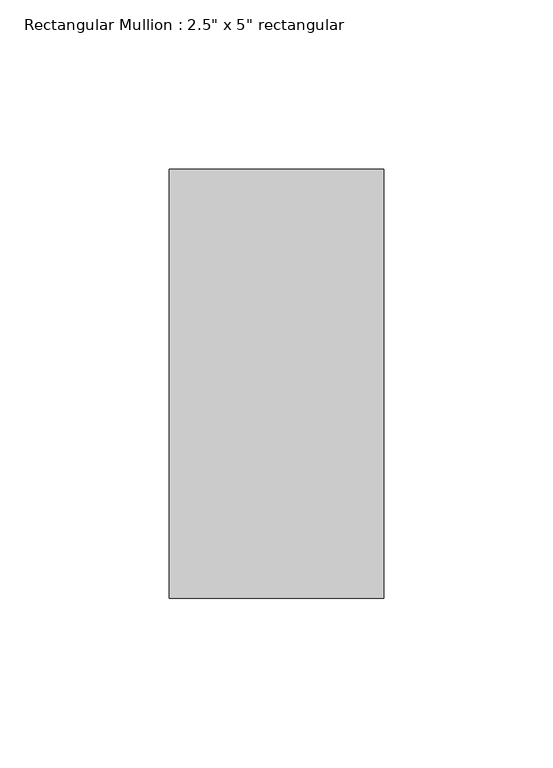
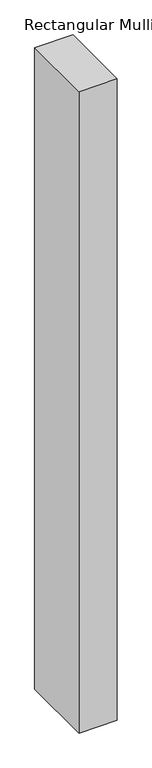
"""IFC4 building model written with IfcOpenShell, lengths in millimetres: member geometry."""

from ifc_helpers import new_model, si_unit, frame, origin, place, context, project, spatial, polyline, outline, extrude, source, transform, mapped, element, save


def member_866a01fa(model_context):
    return source(origin(), model_context, "Body", "SweptSolid", [
        extrude(outline(polyline([(31.75, 63.5), (31.75, -63.5), (-31.75, -63.5), (-31.75, 63.5), (31.75, 63.5)])), frame((0.0, 0.0, -1123.95), z_axis=(0.0, 0.0, 1.0), x_axis=(1.0, 0.0, 0.0)), (0.0, 0.0, 1.0), 1123.95),
    ])


if __name__ == "__main__":
    model = new_model("IFC4")
    model_context = context("Model", 3, world=origin())
    ifc_project = project(units=[si_unit("LENGTHUNIT", "METRE", prefix="MILLI")], contexts=[model_context])
    site = spatial("IfcSite", under=ifc_project)
    building = spatial("IfcBuilding", under=site)
    placement = place(None, origin())
    member_shape = member_866a01fa(model_context)
    element("IfcMember", 1, ObjectType="Rectangular Mullion : 2.5\" x 5\" rectangular", at=placement, inside=building, context=model_context, shape_type="MappedRepresentation", body=[
        mapped(member_shape, transform((0.0, 0.0, 0.0), x_axis=(1.0, 0.0, 0.0), y_axis=(0.0, 1.0, 0.0), z_axis=(0.0, 0.0, 1.0))),
    ])
    save(model, "model.ifc")

# Revit data of these elements
# Type "Rectangular Mullion : 2.5\" x 5\" rectangular"
#   built-in parameter 1007304 = 0.416667 (stored number, unit not read)
#   built-in parameter 1007301 = 0.104167 (stored number, unit not read)
#   built-in parameter 1007300 = 0.104167 (stored number, unit not read)
# Element 1 (IfcMember, "Rectangular Mullion : 2.5\" x 5\" rectangular")
#   Materials on its faces: "Door - Frame"
# Materials
#   "Door - Frame": colour RGB 118 70 51, transparency 0, Cost = 0
